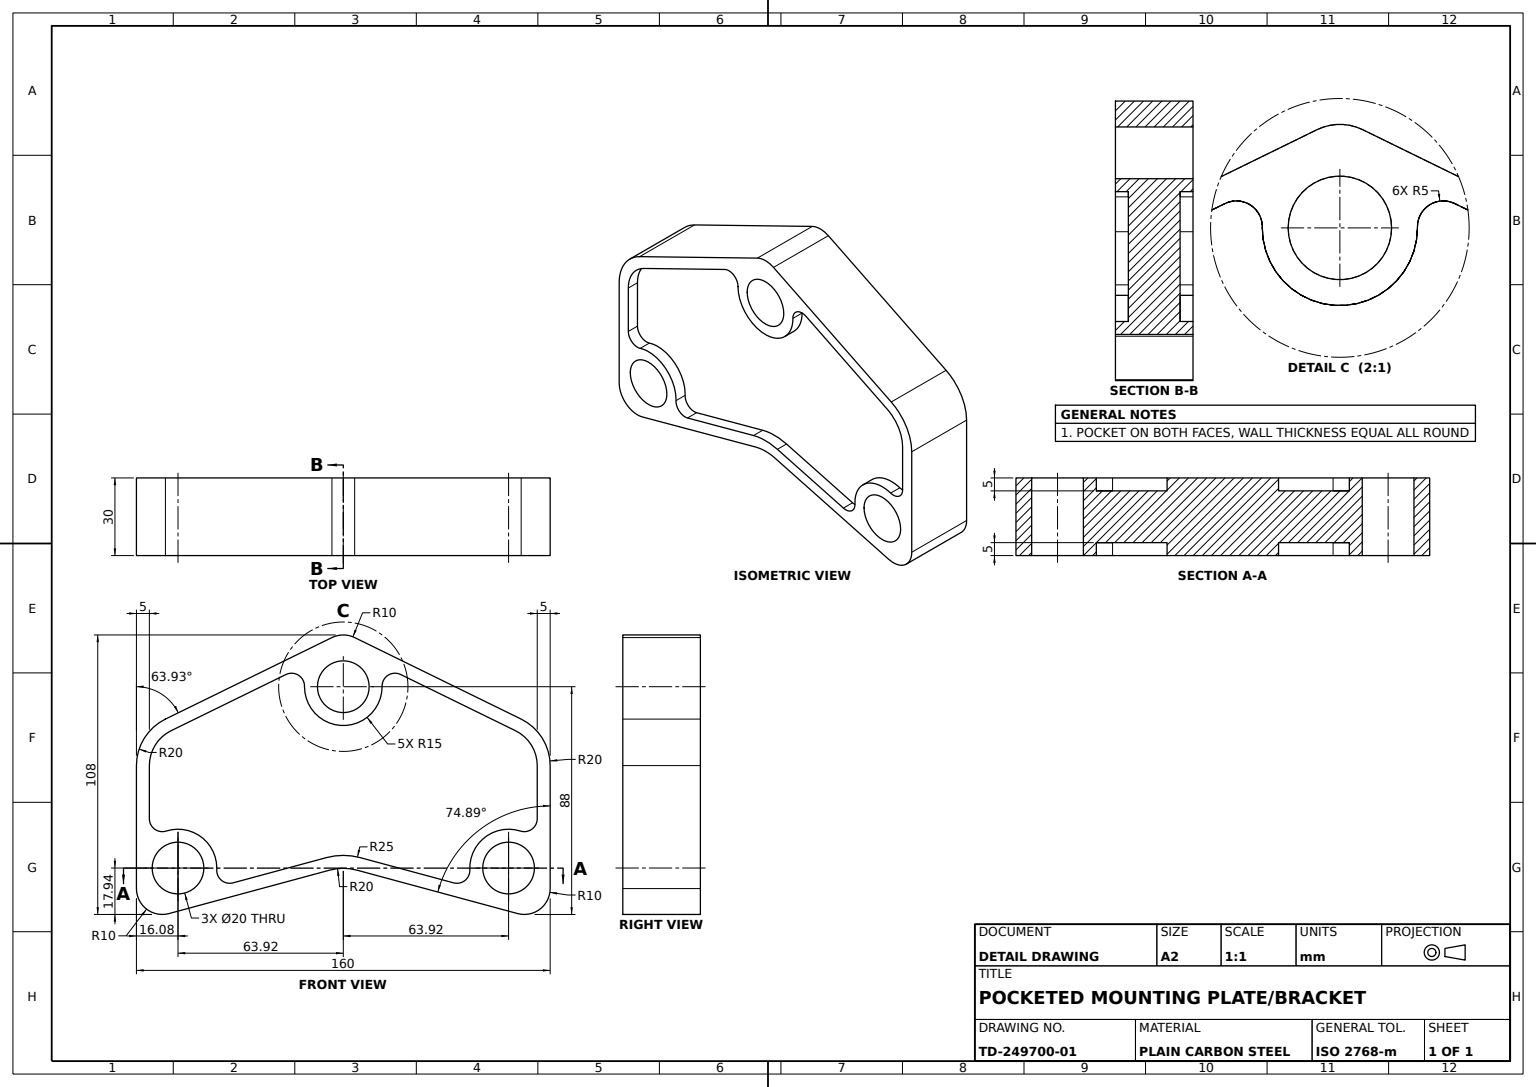
from build123d import *

# Parameters (mm, degrees)
BRACKET_PLATE_DEPTH          = 15
FRONT_FACE_POCKET_DEPTH      = 5
MOUNTING_HOLES_X3_DEPTH      = 129.953479984
MOUNTING_HOLES_X3_DEPTH_BACK = 129.953479984
MOUNTING_HOLES_SKETCH_R      = 10


with BuildPart() as part:
    # Bracket Outline Sketch → Bracket Plate (new, symmetric)
    with BuildSketch(Plane.XY):
        with BuildLine():
            Line((-80, -88), (-80, -40.481444811))
            ThreePointArc((-80, -40.481444811), (-76.967037057, -29.892787979), (-68.78803465, -22.515631526))
            Line((-68.78803465, -22.515631526), (-4.394017325, 8.982906643))
            ThreePointArc((-4.394017325, 8.982906643), (0, 10), (4.394017325, 8.982906643))
            Line((4.394017325, 8.982906643), (68.78803465, -22.515631526))
            ThreePointArc((68.78803465, -22.515631526), (76.967037057, -29.892787979), (80, -40.481444811))
            Line((80, -40.481444811), (80, -88))
            ThreePointArc((80, -88), (76.079830561, -95.939500006), (67.39286793, -97.654162955))
            Line((67.39286793, -97.654162955), (5.21426414, -80.862667644))
            ThreePointArc((5.21426414, -80.862667644), (0, -80.170993555), (-5.21426414, -80.862667644))
            Line((-5.21426414, -80.862667644), (-67.39286793, -97.654162955))
            ThreePointArc((-67.39286793, -97.654162955), (-76.079830561, -95.939500006), (-80, -88))
        make_face()
    extrude(amount=BRACKET_PLATE_DEPTH, both=True)

    # Face Pocket Sketch → Front Face Pocket (cut)
    with BuildSketch(Plane.XY.offset(15)):
        with BuildLine():
            Line((75, -61.007005292), (75, -40.481444811))
            ThreePointArc((75, -40.481444811), (72.725277793, -32.539952187), (66.591025987, -27.007084847))
            Line((66.591025987, -27.007084847), (22.195825808, -5.291031626))
            ThreePointArc((22.195825808, -5.291031626), (17.328625574, -5.555183565), (14.999112859, -9.83686371))
            ThreePointArc((14.999112859, -9.83686371), (0, -25), (-14.999112859, -9.83686371))
            ThreePointArc((-14.999112859, -9.83686371), (-17.328625574, -5.555183565), (-22.195825808, -5.291031626))
            Line((-22.195825808, -5.291031626), (-66.591025987, -27.007084847))
            ThreePointArc((-66.591025987, -27.007084847), (-72.725277793, -32.539952187), (-75, -40.481444811))
            Line((-75, -40.481444811), (-75, -61.007005292))
            ThreePointArc((-75, -61.007005292), (-72.949594192, -65.044318025), (-68.48004236, -65.770378967))
            ThreePointArc((-68.48004236, -65.770378967), (-54.800423598, -68.151249984), (-48.935434642, -80.737052336))
            ThreePointArc((-48.935434642, -80.737052336), (-47.069212384, -84.862736832), (-42.636957008, -85.789651261))
            Line((-42.636957008, -85.789651261), (-6.517830175, -76.035586166))
            ThreePointArc((-6.517830175, -76.035586166), (0, -75.170993555), (6.517830175, -76.035586166))
            Line((6.517830175, -76.035586166), (42.636957008, -85.789651261))
            ThreePointArc((42.636957008, -85.789651261), (47.069212384, -84.862736832), (48.935434642, -80.737052336))
            ThreePointArc((48.935434642, -80.737052336), (54.800423598, -68.151249984), (68.48004236, -65.770378967))
            ThreePointArc((68.48004236, -65.770378967), (72.949594192, -65.044318025), (75, -61.007005292))
        make_face()
    front_face_pocket = extrude(amount=-FRONT_FACE_POCKET_DEPTH, mode=Mode.SUBTRACT)

    # Back Face Pocket Mirror: Front Face Pocket across plane
    add(front_face_pocket.mirror(Plane.XY), mode=Mode.SUBTRACT)

    # Mounting Holes Sketch → Mounting Holes x3 (cut, two sides: drawn at the far end of the back side and taken through both)
    with BuildSketch(Plane.XY.offset(10).offset(-MOUNTING_HOLES_X3_DEPTH_BACK)):
        with Locations((-63.920169439, -80.060499994)):
            Circle(MOUNTING_HOLES_SKETCH_R)
        with Locations((0, -10)):
            Circle(MOUNTING_HOLES_SKETCH_R)
        with Locations((63.920169439, -80.060499994)):
            Circle(MOUNTING_HOLES_SKETCH_R)
    extrude(amount=MOUNTING_HOLES_X3_DEPTH + MOUNTING_HOLES_X3_DEPTH_BACK, mode=Mode.SUBTRACT)


solid = part.part
